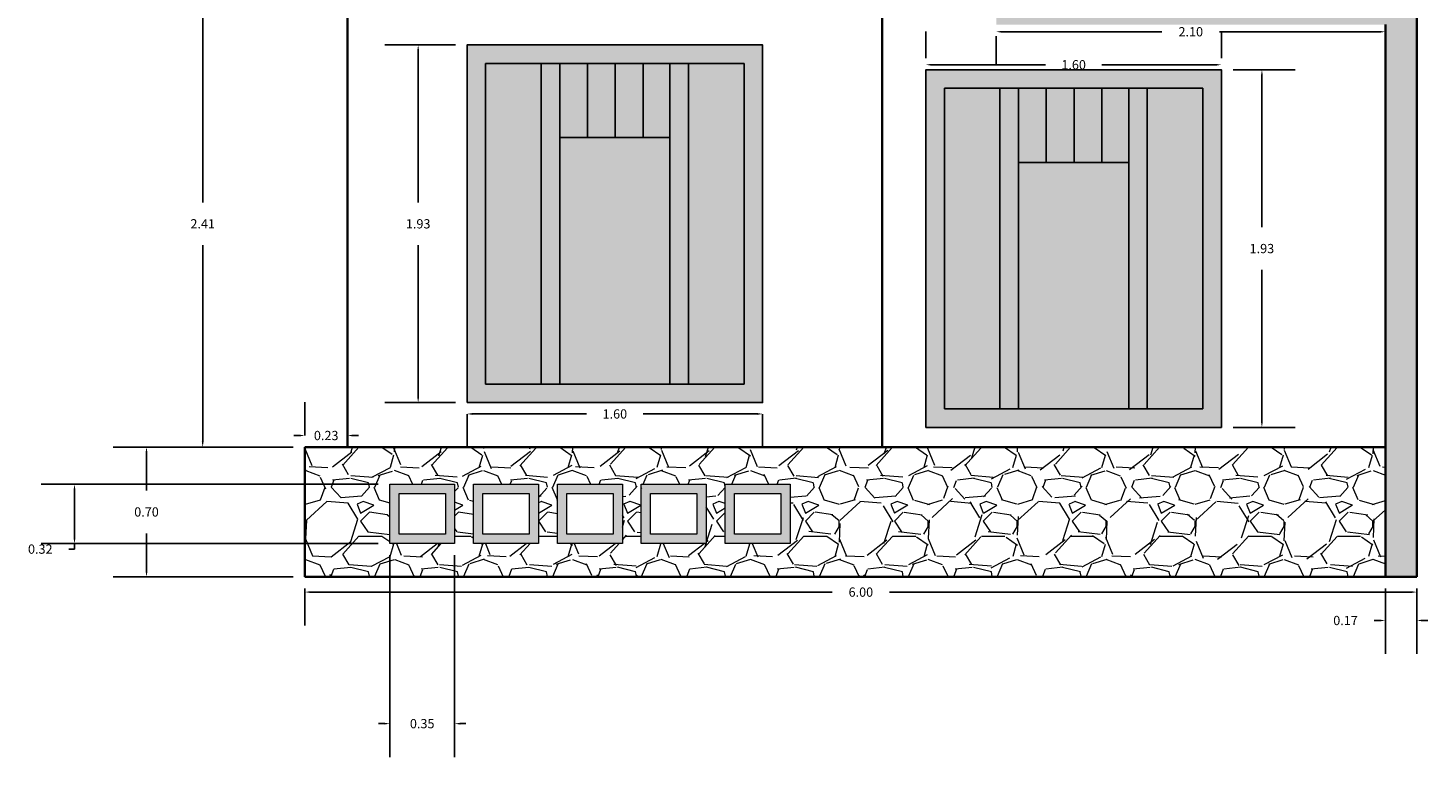
# Model space of a CAD drawing. Units: metres. Extents: x -184.63 to -177.08, y -586.84 to -578.06.
# Tile 1 of 2: x -184.63 to -177.08, y -586.84 to -582.9. Entities that reach past the tile are written whole.
import ezdxf

# ---------------------------------------------------------------- set-up
doc = ezdxf.new("R2010")
doc.units = ezdxf.units.M
doc.header["$MEASUREMENT"] = 0
for name, color, linetype, lineweight in [('A-ANNO-DIMS', 2, 'Continuous', 18), ('A-DOOR', 4, 'Continuous', 25), ('A-ELEV', 7, 'Continuous', 35), ('A-ELEV-PATT', 8, 'Continuous', 13), ('A-GLAZ', 3, 'Continuous', 18)]:
    doc.layers.add(name, color=color, linetype=linetype, lineweight=lineweight)
doc.styles.get("Standard").update_dxf_attribs({"font": 'arial.ttf'})
doc.dimstyles.get("Standard").update_dxf_attribs({"dimtxt": 0.05, "dimasz": 0.03, "dimexe": 0.18, "dimexo": 0.0625, "dimgap": 0.09, "dimtad": 0, "dimtih": 1, "dimtoh": 1, "dimzin": 0, "dimdsep": 46, "dimtxsty": 'Standard', "dimcen": 0.09, "dimadec": 0, "dimazin": 0, "dimtfac": 1, "dimtofl": 0, "dimtmove": 0, "dimatfit": 3, "dimfxl": 1, "dimtolj": 1, "dimtzin": 0, "dimarcsym": 0})

# ---------------------------------------------------------------- blocks, each defined once
blk = doc.blocks.new('*D1')
at = {"layer": 'A-ANNO-DIMS', "color": 0, "lineweight": -2, "transparency": 16777216}
for p, q in [((-183.2004953711962, -585.1641223595374), (-184.1725236562688, -585.1641223595374)), ((-183.9925236562688, -585.1941223595373), (-183.9925236562688, -585.3985937101515)), ((-183.9925236562688, -585.8341223595374), (-183.9925236562688, -585.6296510089237)), ((-183.2004953711962, -585.8641223595375), (-184.1725236562688, -585.8641223595375))]:
    blk.add_line(p, q, dxfattribs=at)
at = {"layer": 'A-ANNO-DIMS', "color": 0, "transparency": 16777216}
for points in [[(-183.9975236562688, -585.1941223595373), (-183.9875236562688, -585.1941223595373), (-183.9925236562688, -585.1641223595374)], [(-183.9975236562688, -585.8341223595374), (-183.9875236562688, -585.8341223595374), (-183.9925236562688, -585.8641223595375)]]:
    blk.add_solid(points, dxfattribs=at)
at = {"layer": 'Defpoints', "color": 0, "transparency": 16777216}
for p in [(-183.9925236562688, -585.1641223595374), (-183.1379953711963, -585.1641223595374), (-183.1379953711963, -585.8641223595375)]:
    blk.add_point(p, dxfattribs=at)
at = {"layer": 'A-ANNO-DIMS', "color": 0, "transparency": 16777216, "insert": (-183.992523656269, -585.5141223595374), "char_height": 0.05, "attachment_point": 5}
blk.add_mtext('\\A1;0.70', dxfattribs=at)
blk = doc.blocks.new('*D2')
at = {"layer": 'A-ANNO-DIMS', "color": 0, "lineweight": -2, "transparency": 16777216}
for p, q in [((-182.9704953711963, -582.7541223595375), (-183.8692916661182, -582.7541223595375)), ((-183.6892916661182, -582.7841223595375), (-183.6892916661182, -583.8440200403014)), ((-183.6892916661182, -585.1341223595375), (-183.6892916661182, -584.0742246787734)), ((-183.2004953711962, -585.1641223595374), (-183.8692916661182, -585.1641223595374))]:
    blk.add_line(p, q, dxfattribs=at)
at = {"layer": 'A-ANNO-DIMS', "color": 0, "transparency": 16777216}
for points in [[(-183.6942916661182, -582.7841223595375), (-183.6842916661182, -582.7841223595375), (-183.6892916661182, -582.7541223595375)], [(-183.6942916661182, -585.1341223595375), (-183.6842916661182, -585.1341223595375), (-183.6892916661182, -585.1641223595374)]]:
    blk.add_solid(points, dxfattribs=at)
at = {"layer": 'Defpoints', "color": 0, "transparency": 16777216}
for p in [(-183.6892916661182, -582.7541223595375), (-182.9079953711963, -582.7541223595375), (-183.1379953711963, -585.1641223595374)]:
    blk.add_point(p, dxfattribs=at)
at = {"layer": 'A-ANNO-DIMS', "color": 0, "transparency": 16777216, "insert": (-183.6892916661183, -583.9591223595373), "char_height": 0.05, "attachment_point": 5}
blk.add_mtext('\\A1;2.41', dxfattribs=at)
blk = doc.blocks.new('*D4')
at = {"layer": 'A-ANNO-DIMS', "color": 0, "lineweight": -2, "transparency": 16777216}
for p, q in [((-182.6800294737008, -585.74714713752), (-182.6800294737008, -586.8364943431044)), ((-182.3300294737008, -585.74714713752), (-182.3300294737008, -586.8364943431044)), ((-182.7100294737008, -586.6564943431044), (-182.7400294737008, -586.6564943431044)), ((-182.3000294737008, -586.6564943431044), (-182.2700294737009, -586.6564943431044))]:
    blk.add_line(p, q, dxfattribs=at)
at = {"layer": 'A-ANNO-DIMS', "color": 0, "transparency": 16777216}
for points in [[(-182.7100294737008, -586.6514943431044), (-182.7100294737008, -586.6614943431044), (-182.6800294737008, -586.6564943431044)], [(-182.3000294737008, -586.6514943431044), (-182.3000294737008, -586.6614943431044), (-182.3300294737008, -586.6564943431044)]]:
    blk.add_solid(points, dxfattribs=at)
at = {"layer": 'Defpoints', "color": 0, "transparency": 16777216}
for p in [(-182.6800294737008, -585.6846471375201), (-182.3300294737008, -585.6846471375201), (-182.3300294737008, -586.6564943431044)]:
    blk.add_point(p, dxfattribs=at)
at = {"layer": 'A-ANNO-DIMS', "color": 0, "transparency": 16777216, "insert": (-182.5050294737008, -586.6564943431044), "char_height": 0.05, "attachment_point": 5}
blk.add_mtext('\\A1;0.35', dxfattribs=at)
blk = doc.blocks.new('*D5')
at = {"layer": 'A-ANNO-DIMS', "color": 0, "lineweight": -2, "transparency": 16777216}
for p, q in [((-182.7425294737009, -585.3646471375203), (-184.5609941601875, -585.3646471375203)), ((-184.3809941601874, -585.3946471375202), (-184.3809941601874, -585.6546471375203)), ((-182.7425294737009, -585.6846471375202), (-184.5609941601875, -585.6846471375202)), ((-184.3809941601874, -585.7146471375203), (-184.4109941601874, -585.7146471375203)), ((-184.3809941601874, -585.6846471375202), (-184.3809941601874, -585.7146471375203))]:
    blk.add_line(p, q, dxfattribs=at)
at = {"layer": 'A-ANNO-DIMS', "color": 0, "transparency": 16777216}
for points in [[(-184.3859941601874, -585.3946471375202), (-184.3759941601875, -585.3946471375202), (-184.3809941601874, -585.3646471375203)], [(-184.3859941601874, -585.6546471375203), (-184.3759941601875, -585.6546471375203), (-184.3809941601874, -585.6846471375202)]]:
    blk.add_solid(points, dxfattribs=at)
at = {"layer": 'Defpoints', "color": 0, "transparency": 16777216}
for p in [(-182.6800294737009, -585.3646471375203), (-184.3809941601874, -585.6846471375202), (-182.6800294737009, -585.6846471375202)]:
    blk.add_point(p, dxfattribs=at)
at = {"layer": 'A-ANNO-DIMS', "color": 0, "transparency": 16777216, "insert": (-184.5656769705559, -585.71464713752), "char_height": 0.05, "attachment_point": 5}
blk.add_mtext('\\A1;0.32', dxfattribs=at)
blk = doc.blocks.new('*D6')
at = {"layer": 'A-ANNO-DIMS', "color": 0, "lineweight": -2, "transparency": 16777216}
for p, q in [((-182.3254953711962, -582.9941223595375), (-182.7066942871716, -582.9941223595375)), ((-182.5266942871716, -583.0241223595375), (-182.5266942871716, -583.8435766569453)), ((-182.5266942871716, -584.8941223595375), (-182.5266942871716, -584.0746680621294)), ((-182.3254953711962, -584.9241223595375), (-182.7066942871716, -584.9241223595375))]:
    blk.add_line(p, q, dxfattribs=at)
at = {"layer": 'A-ANNO-DIMS', "color": 0, "transparency": 16777216}
for points in [[(-182.5316942871716, -583.0241223595375), (-182.5216942871716, -583.0241223595375), (-182.5266942871716, -582.9941223595375)], [(-182.5316942871716, -584.8941223595375), (-182.5216942871716, -584.8941223595375), (-182.5266942871716, -584.9241223595375)]]:
    blk.add_solid(points, dxfattribs=at)
at = {"layer": 'Defpoints', "color": 0, "transparency": 16777216}
for p in [(-182.5266942871716, -582.9941223595375), (-182.2629953711962, -582.9941223595375), (-182.2629953711962, -584.9241223595375)]:
    blk.add_point(p, dxfattribs=at)
at = {"layer": 'A-ANNO-DIMS', "color": 0, "transparency": 16777216, "insert": (-182.5266942871717, -583.9591223595373), "char_height": 0.05, "attachment_point": 5}
blk.add_mtext('\\A1;1.93', dxfattribs=at)
blk = doc.blocks.new('*D7')
at = {"layer": 'A-ANNO-DIMS', "color": 0, "lineweight": -2, "transparency": 16777216}
for p, q in [((-182.2629953711962, -584.9866223595373), (-182.2629953711962, -585.165209521304)), ((-182.2329953711962, -584.9852095213041), (-181.6179953711962, -584.9852095213041)), ((-180.6979953711962, -584.9852095213041), (-181.3129953711962, -584.9852095213041)), ((-180.6679953711962, -584.9866223595373), (-180.6679953711962, -585.165209521304))]:
    blk.add_line(p, q, dxfattribs=at)
at = {"layer": 'A-ANNO-DIMS', "color": 0, "transparency": 16777216}
for points in [[(-182.2329953711962, -584.9802095213041), (-182.2329953711962, -584.9902095213041), (-182.2629953711962, -584.9852095213041)], [(-180.6979953711962, -584.9802095213041), (-180.6979953711962, -584.9902095213041), (-180.6679953711962, -584.9852095213041)]]:
    blk.add_solid(points, dxfattribs=at)
at = {"layer": 'Defpoints', "color": 0, "transparency": 16777216}
for p in [(-182.2629953711962, -584.9241223595373), (-180.6679953711962, -584.9241223595373), (-180.6679953711962, -584.9852095213041)]:
    blk.add_point(p, dxfattribs=at)
at = {"layer": 'A-ANNO-DIMS', "color": 0, "transparency": 16777216, "insert": (-181.4654953711962, -584.9852095213041), "char_height": 0.05, "attachment_point": 5}
blk.add_mtext('\\A1;1.60', dxfattribs=at)
blk = doc.blocks.new('*D8')
at = {"layer": 'A-ANNO-DIMS', "color": 0, "lineweight": -2, "transparency": 16777216}
for p, q in [((-183.1379953711962, -585.1016223595371), (-183.1379953711962, -584.9216223595373)), ((-182.9079953711962, -585.1016223595371), (-182.9079953711962, -584.9216223595373)), ((-183.1679953711962, -585.1016223595371), (-183.1979953711962, -585.1016223595371)), ((-182.8779953711962, -585.1016223595371), (-182.8479953711962, -585.1016223595371))]:
    blk.add_line(p, q, dxfattribs=at)
at = {"layer": 'A-ANNO-DIMS', "color": 0, "transparency": 16777216}
for points in [[(-183.1679953711962, -585.0966223595372), (-183.1679953711962, -585.1066223595373), (-183.1379953711962, -585.1016223595371)], [(-182.8779953711962, -585.0966223595372), (-182.8779953711962, -585.1066223595373), (-182.9079953711962, -585.1016223595371)]]:
    blk.add_solid(points, dxfattribs=at)
at = {"layer": 'Defpoints', "color": 0, "transparency": 16777216}
for p in [(-182.9079953711962, -585.1016223595371), (-183.1379953711962, -585.1641223595371), (-182.9079953711962, -585.1641223595371)]:
    blk.add_point(p, dxfattribs=at)
at = {"layer": 'A-ANNO-DIMS', "color": 0, "transparency": 16777216, "insert": (-183.0229953711962, -585.1016223595371), "char_height": 0.05, "attachment_point": 5}
blk.add_mtext('\\A1;0.23', dxfattribs=at)
blk = doc.blocks.new('*D12')
at = {"layer": 'A-ANNO-DIMS', "color": 0, "lineweight": -2, "transparency": 16777216}
for p, q in [((-178.1299581388774, -583.1276726434131), (-177.7941684930734, -583.1276726434131)), ((-177.9741684930734, -583.157672643413), (-177.9741684930734, -583.977126940821)), ((-177.9741684930734, -585.027672643413), (-177.9741684930734, -584.2082183460051)), ((-178.1299581388774, -585.057672643413), (-177.7941684930734, -585.057672643413))]:
    blk.add_line(p, q, dxfattribs=at)
at = {"layer": 'A-ANNO-DIMS', "color": 0, "transparency": 16777216}
for points in [[(-177.9791684930734, -583.157672643413), (-177.9691684930734, -583.157672643413), (-177.9741684930734, -583.1276726434131)], [(-177.9791684930734, -585.027672643413), (-177.9691684930734, -585.027672643413), (-177.9741684930734, -585.057672643413)]]:
    blk.add_solid(points, dxfattribs=at)
at = {"layer": 'Defpoints', "color": 0, "transparency": 16777216}
for p in [(-178.1924581388774, -583.1276726434131), (-178.1924581388774, -585.057672643413), (-177.9741684930734, -585.057672643413)]:
    blk.add_point(p, dxfattribs=at)
at = {"layer": 'A-ANNO-DIMS', "color": 0, "transparency": 16777216, "insert": (-177.9741684930735, -584.0926726434129), "char_height": 0.05, "attachment_point": 5}
blk.add_mtext('\\A1;1.93', dxfattribs=at)
blk = doc.blocks.new('*D14')
at = {"layer": 'A-ANNO-DIMS', "color": 0, "lineweight": -2, "transparency": 16777216}
for p, q in [((-179.3779953711962, -582.9227502245609), (-178.5132750437746, -582.9227502245609)), ((-177.3379953711962, -582.9227502245609), (-178.2027156986177, -582.9227502245609)), ((-179.4079953711962, -582.9464852889482), (-179.4079953711962, -583.102750224561)), ((-177.3079953711962, -582.9464852889482), (-177.3079953711962, -583.102750224561))]:
    blk.add_line(p, q, dxfattribs=at)
at = {"layer": 'A-ANNO-DIMS', "color": 0, "transparency": 16777216}
for points in [[(-179.3779953711962, -582.917750224561), (-179.3779953711962, -582.9277502245609), (-179.4079953711962, -582.9227502245609)], [(-177.3379953711962, -582.917750224561), (-177.3379953711962, -582.9277502245609), (-177.3079953711962, -582.9227502245609)]]:
    blk.add_solid(points, dxfattribs=at)
at = {"layer": 'Defpoints', "color": 0, "transparency": 16777216}
for p in [(-179.4079953711962, -582.8839852889482), (-177.3079953711962, -582.8839852889482), (-177.3079953711962, -582.9227502245609)]:
    blk.add_point(p, dxfattribs=at)
at = {"layer": 'A-ANNO-DIMS', "color": 0, "transparency": 16777216, "insert": (-178.3579953711962, -582.9227502245609), "char_height": 0.05, "attachment_point": 5}
blk.add_mtext('\\A1;2.10', dxfattribs=at)
blk = doc.blocks.new('*D15')
at = {"layer": 'A-ANNO-DIMS', "color": 0, "lineweight": -2, "transparency": 16777216}
for p, q in [((-179.7874581388773, -583.0651726434129), (-179.7874581388773, -582.9209062459076)), ((-178.1924581388774, -583.0651726434129), (-178.1924581388774, -582.9209062459076)), ((-179.7574581388773, -583.1009062459076), (-179.1424581388773, -583.1009062459076)), ((-178.2224581388773, -583.1009062459076), (-178.8374581388773, -583.1009062459076))]:
    blk.add_line(p, q, dxfattribs=at)
at = {"layer": 'A-ANNO-DIMS', "color": 0, "transparency": 16777216}
for points in [[(-179.7574581388773, -583.0959062459076), (-179.7574581388773, -583.1059062459075), (-179.7874581388773, -583.1009062459076)], [(-178.2224581388773, -583.0959062459076), (-178.2224581388773, -583.1059062459075), (-178.1924581388774, -583.1009062459076)]]:
    blk.add_solid(points, dxfattribs=at)
at = {"layer": 'Defpoints', "color": 0, "transparency": 16777216}
for p in [(-179.7874581388773, -583.1276726434128), (-178.1924581388774, -583.1009062459076), (-178.1924581388774, -583.1276726434128)]:
    blk.add_point(p, dxfattribs=at)
at = {"layer": 'A-ANNO-DIMS', "color": 0, "transparency": 16777216, "insert": (-178.9899581388773, -583.1009062459076), "char_height": 0.05, "attachment_point": 5}
blk.add_mtext('\\A1;1.60', dxfattribs=at)
blk = doc.blocks.new('*D16')
at = {"layer": 'A-ANNO-DIMS', "color": 0, "lineweight": -2, "transparency": 16777216}
for p, q in [((-183.1379953711962, -585.9266223595373), (-183.1379953711962, -586.1265467851359)), ((-183.1079953711962, -585.9465467851359), (-180.2929851392726, -585.9465467851359)), ((-177.1679953711962, -585.9465467851359), (-179.9830056031198, -585.9465467851359)), ((-177.1379953711962, -585.9266223595373), (-177.1379953711962, -586.1265467851359))]:
    blk.add_line(p, q, dxfattribs=at)
at = {"layer": 'A-ANNO-DIMS', "color": 0, "transparency": 16777216}
for points in [[(-183.1079953711962, -585.9415467851359), (-183.1079953711962, -585.9515467851359), (-183.1379953711962, -585.9465467851359)], [(-177.1679953711962, -585.9415467851359), (-177.1679953711962, -585.9515467851359), (-177.1379953711962, -585.9465467851359)]]:
    blk.add_solid(points, dxfattribs=at)
at = {"layer": 'Defpoints', "color": 0, "transparency": 16777216}
for p in [(-183.1379953711962, -585.8641223595372), (-177.1379953711962, -585.8641223595372), (-177.1379953711962, -585.9465467851359)]:
    blk.add_point(p, dxfattribs=at)
at = {"layer": 'A-ANNO-DIMS', "color": 0, "transparency": 16777216, "insert": (-180.1379953711962, -585.9465467851359), "char_height": 0.05, "attachment_point": 5}
blk.add_mtext('\\A1;6.00', dxfattribs=at)
blk = doc.blocks.new('*D17')
at = {"layer": 'A-ANNO-DIMS', "color": 0, "lineweight": -2, "transparency": 16777216}
for p, q in [((-177.3079953711962, -585.9266223595373), (-177.3079953711962, -586.2797984827756)), ((-177.1379953711962, -585.9266223595373), (-177.1379953711962, -586.2797984827756)), ((-177.3379953711962, -586.0997984827756), (-177.3679953711962, -586.0997984827756)), ((-177.1079953711962, -586.0997984827756), (-177.0779953711962, -586.0997984827756))]:
    blk.add_line(p, q, dxfattribs=at)
at = {"layer": 'A-ANNO-DIMS', "color": 0, "transparency": 16777216}
for points in [[(-177.3379953711962, -586.0947984827756), (-177.3379953711962, -586.1047984827755), (-177.3079953711962, -586.0997984827756)], [(-177.1079953711962, -586.0947984827756), (-177.1079953711962, -586.1047984827755), (-177.1379953711962, -586.0997984827756)]]:
    blk.add_solid(points, dxfattribs=at)
at = {"layer": 'Defpoints', "color": 0, "transparency": 16777216}
for p in [(-177.3079953711962, -585.8641223595372), (-177.1379953711962, -585.8641223595372), (-177.3079953711962, -586.0997984827756)]:
    blk.add_point(p, dxfattribs=at)
at = {"layer": 'A-ANNO-DIMS', "color": 0, "transparency": 16777216, "insert": (-177.5229339796546, -586.0997984827756), "char_height": 0.05, "attachment_point": 5}
blk.add_mtext('\\A1;0.17', dxfattribs=at)
blk = doc.blocks.new('VENT')
for points in [[(-179.5064621376118, -580.4941223595374), (-179.1564621376118, -580.4941223595374), (-179.1564621376118, -580.8141223595374), (-179.5064621376118, -580.8141223595374)], [(-179.4564621376117, -580.5441223595373), (-179.2064621376117, -580.5441223595373), (-179.2064621376117, -580.7641223595374), (-179.4564621376117, -580.7641223595374)]]:
    blk.add_lwpolyline(points, close=True)

msp = doc.modelspace()

# ---------------------------------------------------------------- hatches: boundary and pattern name
at = {"layer": 'A-ELEV-PATT'}
h = msp.add_hatch(color=256, dxfattribs=at)
h.dxf.hatch_style = 1
h.set_gradient(color1=(0, 255, 255), color2=(16, 86, 137), name='INVSPHERICAL')
h.paths.add_polyline_path([(-180.9929953711962, -580.2041223595373), (-181.5879953711962, -580.2041223595373), (-181.5879953711962, -581.9041223595372), (-180.9929953711962, -581.9041223595372)])
h.paths.add_polyline_path([(-181.5879953711962, -580.2041223595373), (-181.5879953711962, -579.8041223595372), (-181.6879953711962, -579.8041223595372), (-181.6879953711962, -581.9041223595372), (-181.5879953711962, -581.9041223595372)])
h.paths.add_polyline_path([(-181.6879953711962, -579.8041223595372), (-181.9879953711962, -579.8041223595372), (-181.9879953711962, -581.9041223595372), (-181.6879953711962, -581.9041223595372)])
h.paths.add_polyline_path([(-180.5929953711962, -579.8041223595372), (-180.8929953711962, -579.8041223595372), (-180.8929953711962, -581.9041223595372), (-180.5929953711962, -581.9041223595372)])
h.paths.add_polyline_path([(-180.8929953711962, -579.8041223595372), (-180.9929953711962, -579.8041223595372), (-180.9929953711962, -581.9041223595372), (-180.8929953711962, -581.9041223595372)])
h.paths.add_polyline_path([(-181.4379953711962, -579.8041223595372), (-181.5879953711962, -579.8041223595372), (-181.5879953711962, -580.2041223595373), (-181.4379953711962, -580.2041223595373)])
h.paths.add_polyline_path([(-181.2879953711962, -579.8041223595372), (-181.4379953711962, -579.8041223595372), (-181.4379953711962, -580.2041223595373), (-181.2879953711962, -580.2041223595373)])
h.paths.add_polyline_path([(-180.9929953711962, -579.8041223595372), (-181.1379953711962, -579.8041223595372), (-181.1379953711962, -580.2041223595373), (-180.9929953711962, -580.2041223595373)])
h.paths.add_polyline_path([(-181.1379953711962, -579.8041223595372), (-181.2879953711962, -579.8041223595372), (-181.2879953711962, -580.2041223595373), (-181.1379953711962, -580.2041223595373)])
h.paths.add_polyline_path([(-180.7679953711962, -583.0941223595373), (-181.0679953711962, -583.0941223595373), (-181.0679953711962, -584.8241223595372), (-180.7679953711962, -584.8241223595372)])
h.paths.add_polyline_path([(-181.0679953711962, -583.0941223595373), (-181.1679953711962, -583.0941223595373), (-181.1679953711962, -584.8241223595372), (-181.0679953711962, -584.8241223595372)])
h.paths.add_polyline_path([(-181.8629953711962, -583.0941223595373), (-182.1629953711962, -583.0941223595373), (-182.1629953711962, -584.8241223595372), (-181.8629953711962, -584.8241223595372)])
h.paths.add_polyline_path([(-181.7629953711962, -583.0941223595373), (-181.8629953711962, -583.0941223595373), (-181.8629953711962, -584.8241223595372), (-181.7629953711962, -584.8241223595372)])
h.paths.add_polyline_path([(-181.1679953711962, -583.4941223595373), (-181.7629953711962, -583.4941223595373), (-181.7629953711962, -584.8241223595372), (-181.1679953711962, -584.8241223595372)])
h.paths.add_polyline_path([(-181.6129953711962, -583.0941223595373), (-181.7629953711962, -583.0941223595373), (-181.7629953711962, -583.4941223595373), (-181.6129953711962, -583.4941223595373)])
h.paths.add_polyline_path([(-181.4629953711962, -583.0941223595373), (-181.6129953711962, -583.0941223595373), (-181.6129953711962, -583.4941223595373), (-181.4629953711962, -583.4941223595373)])
h.paths.add_polyline_path([(-181.3129953711962, -583.0941223595373), (-181.4629953711962, -583.0941223595373), (-181.4629953711962, -583.4941223595373), (-181.3129953711962, -583.4941223595373)])
h.paths.add_polyline_path([(-181.1679953711962, -583.0941223595373), (-181.3129953711962, -583.0941223595373), (-181.3129953711962, -583.4941223595373), (-181.1679953711962, -583.4941223595373)])
h.paths.add_polyline_path([(-178.6924581388774, -583.6276726434128), (-179.2874581388773, -583.6276726434128), (-179.2874581388773, -584.9576726434128), (-178.6924581388774, -584.9576726434128)])
h.paths.add_polyline_path([(-179.3874581388773, -583.2276726434129), (-179.6874581388773, -583.2276726434129), (-179.6874581388773, -584.9576726434128), (-179.3874581388773, -584.9576726434128)])
h.paths.add_polyline_path([(-179.2874581388773, -583.6276726434128), (-179.2874581388773, -583.2276726434129), (-179.3874581388773, -583.2276726434129), (-179.3874581388773, -584.9576726434128), (-179.2874581388773, -584.9576726434128)])
h.paths.add_polyline_path([(-179.1374581388773, -583.2276726434129), (-179.2874581388773, -583.2276726434129), (-179.2874581388773, -583.6276726434128), (-179.1374581388773, -583.6276726434128)])
h.paths.add_polyline_path([(-178.9874581388773, -583.2276726434129), (-179.1374581388773, -583.2276726434129), (-179.1374581388773, -583.6276726434128), (-178.9874581388773, -583.6276726434128)])
h.paths.add_polyline_path([(-178.8374581388773, -583.2276726434129), (-178.9874581388773, -583.2276726434129), (-178.9874581388773, -583.6276726434128), (-178.8374581388773, -583.6276726434128)])
h.paths.add_polyline_path([(-178.5924581388774, -583.2276726434129), (-178.6924581388774, -583.2276726434129), (-178.6924581388774, -584.9576726434128), (-178.5924581388774, -584.9576726434128)])
h.paths.add_polyline_path([(-178.6924581388774, -583.2276726434129), (-178.8374581388773, -583.2276726434129), (-178.8374581388773, -583.6276726434128), (-178.6924581388774, -583.6276726434128)])
h.paths.add_polyline_path([(-178.2924581388773, -583.2276726434129), (-178.5924581388774, -583.2276726434129), (-178.5924581388774, -584.9576726434128), (-178.2924581388773, -584.9576726434128)])
h = msp.add_hatch(color=256, dxfattribs=at)
h.dxf.hatch_style = 1
h.paths.add_polyline_path([(-177.1379953711962, -581.6762828319233), (-177.3079953711962, -581.6762828319233), (-177.3079953711962, -581.8839852889482), (-177.3079953711962, -582.8839852889482), (-177.3079953711962, -585.8641223595372), (-177.1379953711962, -585.8641223595372), (-177.1379953711962, -585.1641223595371)])
h = msp.add_hatch(color=256, dxfattribs=at)
h.dxf.hatch_style = 1
h.set_gradient(color1=(0, 0, 255), color2=(0, 255, 255), name='SPHERICAL')
h.paths.add_polyline_path([(-180.6679953711962, -582.9941223595373), (-182.2629953711962, -582.9941223595373), (-182.2629953711962, -584.9241223595373), (-180.6679953711962, -584.9241223595373)])
h.paths.add_polyline_path([(-182.1629953711962, -583.0941223595373), (-180.7679953711962, -583.0941223595373), (-180.7679953711962, -584.8241223595372), (-182.1629953711962, -584.8241223595372)], flags=16)
h.paths.add_polyline_path([(-178.1924581388774, -583.1276726434128), (-179.7874581388773, -583.1276726434128), (-179.7874581388773, -585.0576726434128), (-178.1924581388774, -585.0576726434128)])
h.paths.add_polyline_path([(-178.2924581388773, -583.2276726434129), (-178.2924581388773, -584.9576726434128), (-179.6874581388773, -584.9576726434128), (-179.6874581388773, -583.2276726434129)], flags=16)
h.paths.add_polyline_path([(-177.3079953711962, -581.8839852889482), (-179.4079953711962, -581.8839852889482), (-179.4079953711962, -582.8839852889482), (-177.3079953711962, -582.8839852889482)])
h.paths.add_polyline_path([(-177.4079953711962, -581.9839852889482), (-177.4079953711962, -582.7839852889481), (-179.3079953711962, -582.7839852889481), (-179.3079953711962, -581.9839852889482)], flags=16)
h = msp.add_hatch(dxfattribs=at)
h.set_pattern_fill('GRAVEL', color=256, scale=0.48)
h.set_pattern_definition([(228.012787504, (-182.7923953711962, -585.3841223595373), (-3.840000000000029, -4.320000000000001), [0.06457728, -6.393162262595375]), (184.969740728, (-182.8355953711962, -585.4321223595372), (5.759999999999988, 0.4800000000000168), [0.11081664, -10.97084388539039]), (132.510447078, (-182.9459953711962, -585.4417223595373), (4.800000000000055, -5.279999999999935), [0.07813824, -7.735695646127855]), (267.273689006, (-183.1331953711962, -585.5617223595372), (0.4800000000000117, 9.600000000000009), [0.10091424, -9.990507859981918]), (292.833654178, (-183.1379953711962, -585.6625223595373), (-2.399999999999994, 5.760000000000013), [0.0989544, -9.796499101482382]), (357.273689006, (-183.0995953711962, -585.7537223595373), (-9.600000000000009, 0.4800000000000123), [0.10091424, -9.990507859981918]), (37.6942404667, (-182.9987953711962, -585.7585223595373), (-6.239999999999999, -4.799999999999987), [0.13345392, -13.21192730347968]), (72.2553283749, (-182.8931953711962, -585.6769223595373), (3.360000000000013, 10.56), [0.12599424, -12.47343431847043]), (121.429565615, (-182.8547953711962, -585.5569223595373), (-3.840000000000009, 6.239999999999993), [0.101256, -10.02435509266992]), (175.236358309, (-182.9075953711962, -585.4705223595373), (5.279999999999992, -0.4800000000000182), [0.11559936, -5.664366037820303]), (222.397437798, (-183.0227953711962, -585.4609223595373), (-5.759999999999982, -5.279999999999986), [0.14949504, -14.80002000230155]), (138.814074834, (-182.6579953711962, -585.5665223595373), (-3.360000000000015, 2.879999999999999), [0.05102448, -5.051445510112654]), (171.46923439, (-182.6963953711962, -585.5329223595373), (6.239999999999999, -0.9599999999999976), [0.09707376, -9.61032547975536]), (225, (-182.7923953711962, -585.5185223595372), (-1e-16, -0.4799999999999678), [0.06788208, -0.6109404299390881]), (203.198590514, (-182.8259953711962, -585.4609223595373), (2.399999999999994, 0.959999999999988), [0.03655584, -3.619015250814671]), (291.801409486, (-182.8595953711962, -585.4753223595372), (-0.4799999999998483, 1.440000000000049), [0.05169744, -2.533181667424559]), (30.96375653209999, (-182.8403953711962, -585.5233223595372), (1.440000000000025, 0.9599999999999901), [0.08396592, -2.714890989525743]), (161.565051177, (-182.7683953711962, -585.4801223595372), (0.9600000000000054, -0.4799999999999888), [0.06071568, -1.457177596880831]), (16.389540334, (-183.1379953711962, -585.4753223595372), (4.799999999999983, 1.44000000000002), [0.085056, -8.420565670401311]), (70.3461759419, (-183.0563953711962, -585.4513223595374), (-1.920000000000585, -5.28000000000163), [0.07135728, -7.064355718713119]), (293.198590514, (-182.7683953711962, -585.3841223595373), (-0.9599999999999858, 2.399999999999995), [0.0731112, -3.582459890814671]), (343.610459666, (-182.7395953711962, -585.4513223595374), (-4.799999999999983, 1.44000000000002), [0.085056, -8.420565670401118]), (339.44395478, (-183.1379953711962, -585.7729223595373), (-2.400000000000017, 0.9600000000000116), [0.0820224, -4.019099397752398]), (294.775140569, (-183.0611953711962, -585.8017223595372), (-2.400000000000002, 5.28), [0.06872544, -6.803828670372479]), (66.8014094864, (-182.7635953711962, -585.8641223595372), (0.9599999999999909, 2.399999999999985), [0.0731112, -3.582459890814671]), (17.3540246363, (-182.7347953711962, -585.7969223595373), (-6.239999999999988, -1.919999999999981), [0.08046288, -7.9658033348352]), (69.4439547804, (-182.9987953711962, -585.8641223595372), (-0.9600000000000033, -2.399999999999978), [0.0410112, -4.060110597752398]), (101.309932474, (-182.7923953711962, -585.8641223595372), (-0.4799999999999826, 1.920000000000005), [0.0244752, -2.423054166524543]), (165.963756532, (-182.7971953711962, -585.8401223595373), (1.43999999999998, -0.4800000000000006), [0.0989544, -1.880136300296496]), (186.009005957, (-182.8931953711962, -585.8161223595373), (4.800000000000022, 0.4799999999999919), [0.091704, -9.078683123780545]), (303.690067526, (-182.8403953711962, -585.5665223595373), (-0.4799999999999939, 0.9599999999999932), [0.06922656, -1.661438052222719]), (353.157226587, (-182.8019953711962, -585.6241223595373), (8.160000000000007, -0.9600000000000253), [0.12086112, -11.96523005953358]), (60.9453959009, (-182.6819953711962, -585.6385223595373), (-1.919999999999988, -3.359999999999988), [0.04941888, -4.892483587673759]), (90, (-182.6579953711962, -585.5953223595372), (-0.4799999999999999, 0.48), [0.0288, -0.4512]), (120.256437164, (-182.9027953711962, -585.8017223595372), (1.920000000000004, -3.360000000000003), [0.06668352, -6.601689594935904]), (48.01278750419999, (-182.9363953711962, -585.7441223595373), (3.839999999999999, 4.319999999999987), [0.12915456, -6.328584982595375]), (0, (-182.8499953711962, -585.6481223595372), (0.48, 0.48), [0.1248, -0.3552]), (325.304846469, (-182.7251953711962, -585.6481223595372), (4.800000000000066, -3.359999999999915), [0.07589472, -7.513571664404159]), (254.0546040990001, (-182.6627953711962, -585.6913223595373), (-0.4800000000000181, -1.920000000000002), [0.06988896, -3.424563786854639]), (207.645975364, (-182.6819953711962, -585.7585223595373), (-9.119999999999976, -4.800000000000022), [0.1137912, -11.26534760748451]), (175.42607874, (-182.7827953711962, -585.8113223595371), (-6.239999999999978, 0.4800000000000006), [0.12038352, -11.91795523582507])])
h.paths.add_polyline_path([(-177.3079953711962, -585.1641223595371), (-183.1379953711962, -585.1641223595371), (-183.1379953711962, -585.8641223595372), (-177.3079953711962, -585.8641223595372)])
h.paths.add_polyline_path([(-180.5201301271536, -585.6846471375201), (-180.8701301271536, -585.6846471375201), (-180.8701301271536, -585.36464713752), (-180.5201301271536, -585.36464713752)], flags=16)
h.paths.add_polyline_path([(-180.5701301271536, -585.41464713752), (-180.5701301271536, -585.6346471375201), (-180.8201301271536, -585.6346471375201), (-180.8201301271536, -585.41464713752)], flags=0)
h.paths.add_polyline_path([(-180.9726049637904, -585.6846471375201), (-181.3226049637904, -585.6846471375201), (-181.3226049637904, -585.36464713752), (-180.9726049637904, -585.36464713752)], flags=16)
h.paths.add_polyline_path([(-181.0226049637904, -585.41464713752), (-181.0226049637904, -585.6346471375201), (-181.2726049637904, -585.6346471375201), (-181.2726049637904, -585.41464713752)], flags=0)
h.paths.add_polyline_path([(-181.4250798004272, -585.6846471375201), (-181.7750798004272, -585.6846471375201), (-181.7750798004272, -585.36464713752), (-181.4250798004272, -585.36464713752)], flags=16)
h.paths.add_polyline_path([(-181.4750798004272, -585.41464713752), (-181.4750798004272, -585.6346471375201), (-181.7250798004272, -585.6346471375201), (-181.7250798004272, -585.41464713752)], flags=0)
h.paths.add_polyline_path([(-181.877554637064, -585.6846471375201), (-182.227554637064, -585.6846471375201), (-182.227554637064, -585.36464713752), (-181.877554637064, -585.36464713752)], flags=16)
h.paths.add_polyline_path([(-181.927554637064, -585.41464713752), (-181.927554637064, -585.6346471375201), (-182.177554637064, -585.6346471375201), (-182.177554637064, -585.41464713752)], flags=0)
h.paths.add_polyline_path([(-182.3300294737008, -585.6846471375201), (-182.6800294737008, -585.6846471375201), (-182.6800294737008, -585.36464713752), (-182.3300294737008, -585.36464713752)], flags=16)
h.paths.add_polyline_path([(-182.3800294737009, -585.41464713752), (-182.3800294737009, -585.6346471375201), (-182.6300294737008, -585.6346471375201), (-182.6300294737008, -585.41464713752)], flags=0)
h = msp.add_hatch(color=256, dxfattribs=at)
h.dxf.hatch_style = 1
h.set_gradient(color1=(0, 255, 255), color2=(0, 0, 255), name='INVCYLINDER')
h.paths.add_polyline_path([(-182.3800294737009, -585.41464713752), (-182.6300294737008, -585.41464713752), (-182.6300294737008, -585.6346471375201), (-182.3800294737009, -585.6346471375201)], flags=0)
h.paths.add_polyline_path([(-181.927554637064, -585.41464713752), (-182.177554637064, -585.41464713752), (-182.177554637064, -585.6346471375201), (-181.927554637064, -585.6346471375201)], flags=0)
h.paths.add_polyline_path([(-181.4750798004272, -585.41464713752), (-181.7250798004272, -585.41464713752), (-181.7250798004272, -585.6346471375201), (-181.4750798004272, -585.6346471375201)], flags=0)
h.paths.add_polyline_path([(-181.0226049637904, -585.41464713752), (-181.2726049637904, -585.41464713752), (-181.2726049637904, -585.6346471375201), (-181.0226049637904, -585.6346471375201)], flags=0)
h.paths.add_polyline_path([(-180.5701301271536, -585.41464713752), (-180.8201301271536, -585.41464713752), (-180.8201301271536, -585.6346471375201), (-180.5701301271536, -585.6346471375201)], flags=0)
h.paths.add_polyline_path([(-182.3300294737008, -585.36464713752), (-182.6800294737008, -585.36464713752), (-182.6800294737008, -585.6846471375201), (-182.3300294737008, -585.6846471375201)])
h.paths.add_polyline_path([(-182.6300294737008, -585.6346471375201), (-182.6300294737008, -585.41464713752), (-182.3800294737009, -585.41464713752), (-182.3800294737009, -585.6346471375201)], flags=16)
h.paths.add_polyline_path([(-180.5201301271536, -585.36464713752), (-180.8701301271536, -585.36464713752), (-180.8701301271536, -585.6846471375201), (-180.5201301271536, -585.6846471375201)])
h.paths.add_polyline_path([(-180.5701301271536, -585.41464713752), (-180.5701301271536, -585.6346471375201), (-180.8201301271536, -585.6346471375201), (-180.8201301271536, -585.41464713752)], flags=16)
h.paths.add_polyline_path([(-180.9726049637904, -585.36464713752), (-181.3226049637904, -585.36464713752), (-181.3226049637904, -585.6846471375201), (-180.9726049637904, -585.6846471375201)])
h.paths.add_polyline_path([(-181.0226049637904, -585.41464713752), (-181.0226049637904, -585.6346471375201), (-181.2726049637904, -585.6346471375201), (-181.2726049637904, -585.41464713752)], flags=16)
h.paths.add_polyline_path([(-181.4250798004272, -585.36464713752), (-181.7750798004272, -585.36464713752), (-181.7750798004272, -585.6846471375201), (-181.4250798004272, -585.6846471375201)])
h.paths.add_polyline_path([(-181.4750798004272, -585.41464713752), (-181.4750798004272, -585.6346471375201), (-181.7250798004272, -585.6346471375201), (-181.7250798004272, -585.41464713752)], flags=16)
h.paths.add_polyline_path([(-181.877554637064, -585.36464713752), (-182.227554637064, -585.36464713752), (-182.227554637064, -585.6846471375201), (-181.877554637064, -585.6846471375201)])
h.paths.add_polyline_path([(-181.927554637064, -585.41464713752), (-181.927554637064, -585.6346471375201), (-182.177554637064, -585.6346471375201), (-182.177554637064, -585.41464713752)], flags=16)

# ---------------------------------------------------------------- linework, layer by layer
at = {"layer": 'A-DOOR'}
for p, q in [((-182.1629953711962, -584.8241223595372), (-182.1629953711962, -583.0941223595373)), ((-182.1629953711962, -583.0941223595373), (-180.7679953711962, -583.0941223595373)), ((-181.8629953711962, -584.8241223595372), (-181.8629953711962, -583.0941223595373)), ((-181.7629953711962, -584.8241223595372), (-181.7629953711962, -583.0941223595373)), ((-181.6129953711962, -583.4941223595373), (-181.6129953711962, -583.0941223595373)), ((-181.4629953711962, -583.4941223595373), (-181.4629953711962, -583.0941223595373)), ((-181.3129953711962, -583.4941223595373), (-181.3129953711962, -583.0941223595373)), ((-181.1679953711962, -583.0941223595373), (-181.1679953711962, -584.8241223595372)), ((-181.0679953711962, -583.0941223595373), (-181.0679953711962, -584.8241223595372)), ((-180.7679953711962, -583.0941223595373), (-180.7679953711962, -584.8241223595372)), ((-179.6874581388773, -584.9576726434128), (-179.6874581388773, -583.2276726434129)), ((-179.6874581388773, -583.2276726434129), (-178.2924581388773, -583.2276726434129)), ((-179.3874581388773, -584.9576726434128), (-179.3874581388773, -583.2276726434129)), ((-179.2874581388773, -584.9576726434128), (-179.2874581388773, -583.2276726434129)), ((-179.1374581388773, -583.6276726434128), (-179.1374581388773, -583.2276726434129)), ((-178.9874581388773, -583.6276726434128), (-178.9874581388773, -583.2276726434129)), ((-178.8374581388773, -583.6276726434128), (-178.8374581388773, -583.2276726434129)), ((-178.6924581388774, -583.2276726434129), (-178.6924581388774, -584.9576726434128)), ((-178.5924581388774, -583.2276726434129), (-178.5924581388774, -584.9576726434128)), ((-178.2924581388773, -583.2276726434129), (-178.2924581388773, -584.9576726434128)), ((-181.7629953711962, -583.4941223595373), (-181.1679953711962, -583.4941223595373)), ((-179.2874581388773, -583.6276726434128), (-178.6924581388774, -583.6276726434128)), ((-180.7679953711962, -584.8241223595372), (-182.1629953711962, -584.8241223595372)), ((-178.2924581388773, -584.9576726434128), (-179.6874581388773, -584.9576726434128))]:
    msp.add_line(p, q, dxfattribs=at)
for points in [[(-182.2629953711962, -584.9241223595373), (-182.2629953711962, -582.9941223595373), (-180.6679953711962, -582.9941223595373), (-180.6679953711962, -584.9241223595373)], [(-179.7874581388773, -585.0576726434128), (-179.7874581388773, -583.1276726434128), (-178.1924581388774, -583.1276726434128), (-178.1924581388774, -585.0576726434128)]]:
    msp.add_lwpolyline(points, close=True, dxfattribs=at)
at = {"layer": 'A-ELEV'}
for p, q in [((-180.0229953711962, -585.1641223595371), (-180.0229953711962, -578.9541223595373)), ((-177.1379953711962, -578.9541223595373), (-177.1379953711962, -585.1641223595371)), ((-182.9079953711962, -585.1641223595371), (-182.9079953711962, -582.7541223595373)), ((-177.3079953711962, -585.8641223595372), (-177.3079953711962, -582.8839852889482)), ((-177.3079953711962, -585.1641223595371), (-183.1379953711962, -585.1641223595371)), ((-183.1379953711962, -585.1641223595371), (-183.1379953711962, -585.8641223595372)), ((-177.1379953711962, -585.8641223595372), (-177.1379953711962, -585.1641223595371)), ((-183.1379953711962, -585.8641223595372), (-177.1379953711962, -585.8641223595372))]:
    msp.add_line(p, q, dxfattribs=at)

# ---------------------------------------------------------------- block references
at = {"layer": 'A-GLAZ'}
for p in [(-3.173567336209345, -4.870524777945547), (-2.721092499612637, -4.870524777933155), (-2.721092499612637, -4.870524777933155), (-2.268617662935753, -4.870524777945547), (-1.816142826298943, -4.870524777945547), (-1.363667989662161, -4.870524777945547)]:
    msp.add_blockref('VENT', p, dxfattribs=at)

# ---------------------------------------------------------------- dimensions: what is measured, and where the dimension line sits
at = {"layer": 'A-ANNO-DIMS'}
for base, p1, p2, override, picture, middle in [((-183.6892916661182, -582.7541223595375), (-183.1379953711962, -585.1641223595371), (-182.9079953711962, -582.7541223595373), {"dimclrd": 0, "dimclre": 0, "dimclrt": 0, "dimtmove": 1}, '*D2', (-183.6892916661183, -583.9591223595373)), ((-182.5266942871716, -582.9941223595375), (-182.2629953711962, -584.9241223595373), (-182.2629953711962, -582.9941223595373), {"dimclrd": 0, "dimclre": 0, "dimclrt": 0}, '*D6', (-182.5266942871717, -583.9591223595373)), ((-177.9741684930734, -585.057672643413), (-178.1924581388774, -583.1276726434128), (-178.1924581388774, -585.0576726434128), {"dimclrd": 0, "dimclre": 0, "dimclrt": 0}, '*D12', (-177.9741684930735, -584.0926726434129)), ((-184.3809941601874, -585.6846471375202), (-182.6800294737008, -585.36464713752), (-182.6800294737008, -585.6846471375201), {"dimclrd": 0, "dimclre": 0, "dimclrt": 0}, '*D5', (-184.5656769705559, -585.71464713752))]:
    dim = msp.add_linear_dim(base=base, p1=p1, p2=p2, angle=90, dimstyle='Standard', override=override, dxfattribs=at)
    dim.commit()
    dim.dimension.update_dxf_attribs({"geometry": picture, "text_midpoint": middle})
for base, p1, p2, picture, middle in [((-178.1924581388774, -583.1009062459076), (-179.7874581388773, -583.1276726434128), (-178.1924581388774, -583.1276726434128), '*D15', (-178.9899581388773, -583.1009062459076)), ((-182.9079953711962, -585.1016223595371), (-183.1379953711962, -585.1641223595371), (-182.9079953711962, -585.1641223595371), '*D8', (-183.0229953711962, -585.1016223595371))]:
    dim = msp.add_linear_dim(base=base, p1=p1, p2=p2, dimstyle='Standard', override={"dimclrd": 0, "dimclre": 0, "dimclrt": 0}, dxfattribs=at)
    dim.commit()
    dim.dimension.update_dxf_attribs({"geometry": picture, "text_midpoint": middle, "dimtype": 160})
for base, p1, p2, picture, middle in [((-177.3079953711962, -582.9227502245609), (-179.4079953711962, -582.8839852889482), (-177.3079953711962, -582.8839852889482), '*D14', (-178.3579953711962, -582.9227502245609)), ((-180.6679953711962, -584.9852095213041), (-182.2629953711962, -584.9241223595373), (-180.6679953711962, -584.9241223595373), '*D7', (-181.4654953711962, -584.9852095213041)), ((-182.3300294737008, -586.6564943431044), (-182.6800294737008, -585.6846471375201), (-182.3300294737008, -585.6846471375201), '*D4', (-182.5050294737008, -586.6564943431044)), ((-177.1379953711962, -585.9465467851359), (-183.1379953711962, -585.8641223595372), (-177.1379953711962, -585.8641223595372), '*D16', (-180.1379953711962, -585.9465467851359)), ((-177.3079953711962, -586.0997984827756), (-177.1379953711962, -585.8641223595372), (-177.3079953711962, -585.8641223595372), '*D17', (-177.5229339796546, -586.0997984827756))]:
    dim = msp.add_linear_dim(base=base, p1=p1, p2=p2, dimstyle='Standard', override={"dimclrd": 0, "dimclre": 0, "dimclrt": 0}, dxfattribs=at)
    dim.commit()
    dim.dimension.update_dxf_attribs({"geometry": picture, "text_midpoint": middle})
dim = msp.add_linear_dim(base=(-183.9925236562688, -585.1641223595374), p1=(-183.1379953711962, -585.8641223595372), p2=(-183.1379953711962, -585.1641223595371), angle=90, dimstyle='Standard', override={"dimclrd": 0, "dimclre": 0, "dimclrt": 0}, dxfattribs=at)
dim.commit()
dim.dimension.update_dxf_attribs({"geometry": '*D1', "text_midpoint": (-183.992523656269, -585.5141223595374), "dimtype": 160})

doc.saveas('drawing.dxf')
